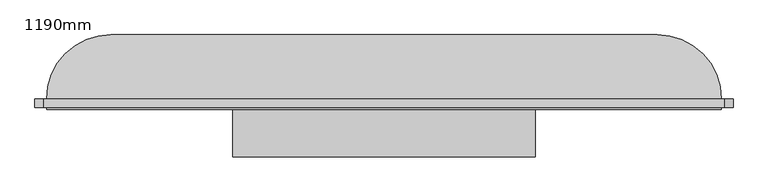
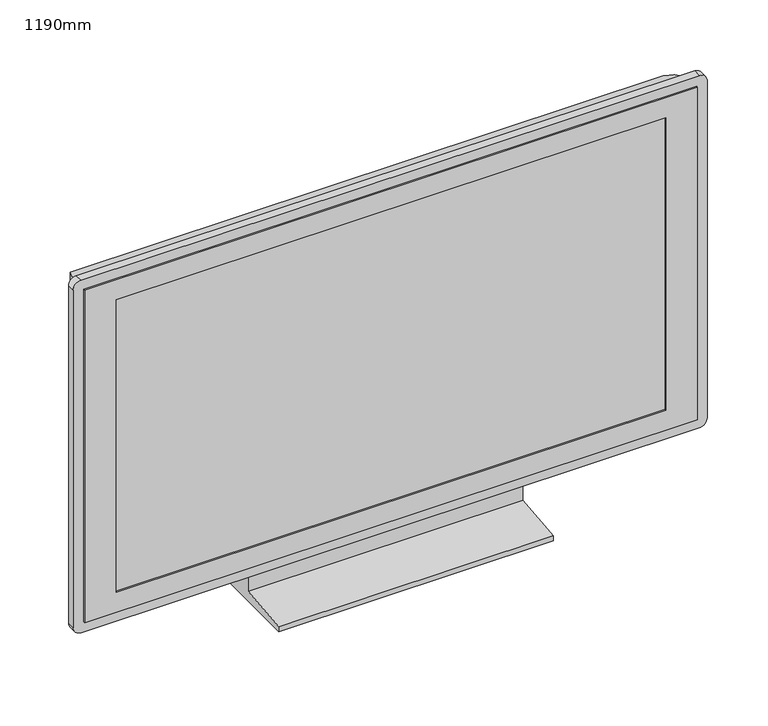
"""IFC4 building model written with IfcOpenShell, lengths in millimetres: furniture geometry, 1190mm."""

from ifc_helpers import new_model, si_unit, point, frame, frame_2d, origin, place, context, project, spatial, polyline, circle_curve, ellipse_curve, trimmed, segment, composite_curve, outline, extrude, faceted_brep, source, transform, mapped, element, save
from ifc_brep_helpers import plane_surface, cylinder_surface, advanced_brep


def furniture_1190mm_d9bcc661(model_context):
    return source(origin(), model_context, "Body", "SolidModel", [
        extrude(outline(polyline([(-51.4613764, 80.0), (-1.4613764, 80.0), (48.5386236, 0.0), (-151.4613764, 0.0), (-151.4613764, 10.0), (-51.4613764, 20.0), (-51.4613764, 80.0)])), frame((-263.2325176, 0.0, 0.0), z_axis=(1.0, 0.0, 0.0), x_axis=(0.0, 1.0, 0.0)), (0.0, 0.0, 1.0), 518.576007),
        faceted_brep([(574.6314928, -69.4613764, 743.4515403), (-582.5205211, -69.4613764, 743.4515403), (-582.5205211, -69.4613764, 80.0), (574.6314928, -69.4613764, 80.0), (-522.5205211, -69.4613764, 703.4515403), (514.6314928, -69.4613764, 703.4515403), (514.6314928, -69.4613764, 120.0), (-522.5205211, -69.4613764, 120.0), (574.6314928, -51.4613764, 743.4515403), (574.6314928, -51.4613764, 80.0), (-582.5205211, -51.4613764, 80.0), (-582.5205211, -51.4613764, 743.4515403), (-522.5205211, -66.4613764, 703.4515403), (-522.5205211, -66.4613764, 120.0), (514.6314928, -66.4613764, 120.0), (514.6314928, -66.4613764, 703.4515403)], [[[0, 1, 2, 3], [4, 5, 6, 7]], [[8, 9, 10, 11]], [[1, 0, 8, 11]], [[2, 1, 11, 10]], [[3, 2, 10, 9]], [[0, 3, 9, 8]], [[12, 13, 14, 15]], [[12, 15, 5, 4]], [[15, 14, 6, 5]], [[14, 13, 7, 6]], [[13, 12, 4, 7]]]),
        extrude(outline(composite_curve([segment(polyline([(763.4515403, 579.6314928), (763.4515403, -587.5205211)]), True, "CONTINUOUS"), segment(trimmed(circle_curve(frame_2d((748.4515403, -587.5205211)), 15.0), [point((763.4515403, -587.5205211))], [point((748.4515403, -602.5205211))], False, "CARTESIAN"), True, "CONTINUOUS"), segment(polyline([(748.4515403, -602.5205211), (75.0, -602.5205211)]), True, "CONTINUOUS"), segment(trimmed(circle_curve(frame_2d((75.0, -587.5205211)), 15.0), [point((75.0, -602.5205211))], [point((60.0, -587.5205211))], False, "CARTESIAN"), True, "CONTINUOUS"), segment(polyline([(60.0, -587.5205211), (60.0, 579.6314928)]), True, "CONTINUOUS"), segment(trimmed(circle_curve(frame_2d((75.0, 579.6314928)), 15.0), [point((60.0, 579.6314928))], [point((75.0, 594.6314928))], False, "CARTESIAN"), True, "CONTINUOUS"), segment(polyline([(75.0, 594.6314928), (748.4515403, 594.6314928)]), True, "CONTINUOUS"), segment(trimmed(circle_curve(frame_2d((748.4515403, 579.6314928)), 15.0), [point((748.4515403, 594.6314928))], [point((763.4515403, 579.6314928))], False, "CARTESIAN"), True, "CONTINUOUS")], self_intersect=False), holes=[polyline([(743.4515403, 574.6314928), (80.0, 574.6314928), (80.0, -582.5205211), (743.4515403, -582.5205211), (743.4515403, 574.6314928)])]), frame((0.0, -66.4613764, 0.0), z_axis=(0.0, 1.0, 0.0), x_axis=(0.0, 0.0, 1.0)), (0.0, 0.0, 1.0), 15.0),
        advanced_brep(
        [(-582.5205211, -51.4613764, 80.0), (574.6314928, -51.4613764, 80.0), (574.6314928, -51.4613764, 743.4515403), (-582.5205211, -51.4613764, 743.4515403), (464.6314928, 58.5386236, 80.0), (-472.5205211, 58.5386236, 80.0), (-472.5205211, 58.5386236, 633.4515403), (464.6314928, 58.5386236, 633.4515403)],
        [
            (0, 1),
            (1, 2),
            (2, 3),
            (3, 0),
            (4, 5),
            (5, 6),
            (6, 7),
            (7, 4),
            (0, 5, circle_curve(frame((-472.5205211, -51.4613764, 80.0), z_axis=(0.0, 0.0, -1.0), x_axis=(-1.0, 0.0, 0.0)), 110.0)),
            (4, 1, circle_curve(frame((464.6314928, -51.4613764, 80.0), z_axis=(0.0, 0.0, -1.0), x_axis=(1.0, 0.0, 0.0)), 110.0)),
            (7, 2, ellipse_curve(frame((464.6314928, -51.4613764, 633.4515403), z_axis=(0.7071067811865475, 0.0, -0.7071067811865475), x_axis=(0.7071067811865474, 0.0, 0.7071067811865476)), 155.5634919, 110.0)),
            (6, 3, ellipse_curve(frame((-472.5205211, -51.4613764, 633.4515403), z_axis=(0.7071067811865475, 0.0, 0.7071067811865476), x_axis=(-0.7071067811865476, 0.0, 0.7071067811865475)), 155.5634919, 110.0)),
        ],
        [
            plane_surface(frame((-582.5205211, -51.4613764, 743.4515403), z_axis=(0.0, -1.0, 0.0), x_axis=(-1.0, 0.0, 0.0))),
            plane_surface(frame((-582.5205211, 58.5386236, 743.4515403), z_axis=(0.0, 1.0, 0.0), x_axis=(1.0, 0.0, 0.0))),
            plane_surface(frame((-582.5205211, -51.4613764, 80.0), z_axis=(0.0, 0.0, -1.0), x_axis=(0.0, 1.0, 0.0))),
            cylinder_surface(frame((464.6314928, -51.4613764, 80.0), z_axis=(0.0, 0.0, 1.0), x_axis=(1.0, 0.0, 0.0)), 110.0),
            cylinder_surface(frame((574.6314928, -51.4613764, 633.4515403), z_axis=(-1.0, 0.0, 0.0), x_axis=(0.0, 0.0, 1.0)), 110.0),
            cylinder_surface(frame((-472.5205211, -51.4613764, 743.4515403), z_axis=(0.0, 0.0, -1.0), x_axis=(-1.0, 0.0, 0.0)), 110.0),
        ],
        [
            (0, [[1, 2, 3, 4]]),
            (1, [[5, 6, 7, 8]]),
            (2, [[-1, 9, -5, 10]]),
            (3, [[11, -2, -10, -8]]),
            (4, [[-11, -7, 12, -3]]),
            (5, [[-12, -6, -9, -4]]),
        ],
    ),
    ])


if __name__ == "__main__":
    model = new_model("IFC4")
    model_context = context("Model", 3, world=origin())
    ifc_project = project(units=[si_unit("LENGTHUNIT", "METRE", prefix="MILLI")], contexts=[model_context])
    site = spatial("IfcSite", under=ifc_project)
    building = spatial("IfcBuilding", under=site)
    placement = place(None, origin())
    furniture_1190mm_shape = furniture_1190mm_d9bcc661(model_context)
    element("IfcFurniture", 1, ObjectType="1190mm", at=placement, inside=building, context=model_context, shape_type="MappedRepresentation", body=[
        mapped(furniture_1190mm_shape, transform((0.0, 0.0, 0.0), x_axis=(1.0, 0.0, 0.0), y_axis=(0.0, 1.0, 0.0), z_axis=(0.0, 0.0, 1.0))),
    ])
    save(model, "model.ifc")

# Revit data of these elements
# Type "1190mm"
#   SinAng = 0.49 mm
#   L = 1037.152 mm
#   H = 583.452 mm
#   Thickness = 110 mm
#   Diagonal = 1190 mm
#   CosAng = 0.872 mm
#   Stand [instance default] = yes
#   Default Elevation = 0
# Element 1 (IfcFurniture, "1190mm")
#   Materials on its faces: "TV - Black", "TV - Glass", "TV - Screen"
# Materials
#   "TV - Black": colour RGB 49 49 49, transparency 0
#   "TV - Glass": colour RGB 157 157 157, transparency 0.9
#   "TV - Screen": colour RGB 0 0 0, transparency 0
